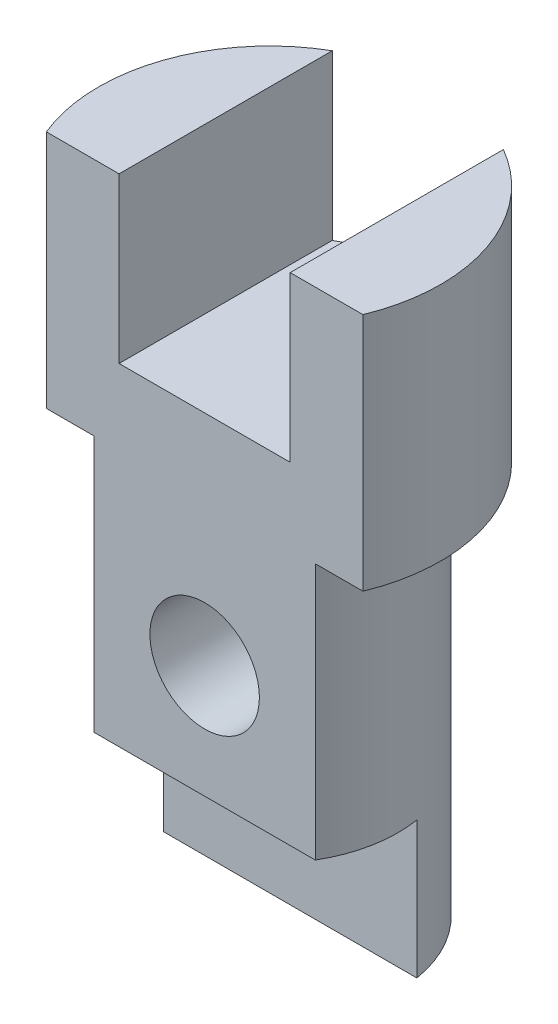
ISO-10303-21;
HEADER;
FILE_DESCRIPTION(('STEP AP214'),'2;1');
FILE_NAME('part.step','',(''),(''),'','','');
FILE_SCHEMA(('AUTOMOTIVE_DESIGN { 1 0 10303 214 1 1 1 1 }'));
ENDSEC;
DATA;
#1=APPLICATION_CONTEXT('core data for automotive mechanical design processes');
#2=APPLICATION_PROTOCOL_DEFINITION('international standard','automotive_design',2000,#1);
#3=PRODUCT_CONTEXT('',#1,'mechanical');
#4=PRODUCT('Part','Part','',(#3));
#5=PRODUCT_RELATED_PRODUCT_CATEGORY('part','',(#4));
#6=PRODUCT_DEFINITION_FORMATION('','',#4);
#7=PRODUCT_DEFINITION_CONTEXT('part definition',#1,'design');
#8=PRODUCT_DEFINITION('design','',#6,#7);
#9=PRODUCT_DEFINITION_SHAPE('','',#8);
#10=(LENGTH_UNIT() NAMED_UNIT(*) SI_UNIT(.MILLI.,.METRE.));
#11=(NAMED_UNIT(*) PLANE_ANGLE_UNIT() SI_UNIT($,.RADIAN.));
#12=(NAMED_UNIT(*) SI_UNIT($,.STERADIAN.) SOLID_ANGLE_UNIT());
#13=UNCERTAINTY_MEASURE_WITH_UNIT(LENGTH_MEASURE(1.E-05),#10,'distance_accuracy_value','');
#14=(GEOMETRIC_REPRESENTATION_CONTEXT(3) GLOBAL_UNCERTAINTY_ASSIGNED_CONTEXT((#13)) GLOBAL_UNIT_ASSIGNED_CONTEXT((#10,
#11,#12)) REPRESENTATION_CONTEXT('',''));
#15=CARTESIAN_POINT('',(0.,0.,0.));
#16=DIRECTION('',(0.,0.,1.));
#17=DIRECTION('',(1.,0.,0.));
#18=AXIS2_PLACEMENT_3D('',#15,#16,#17);
#19=CARTESIAN_POINT('',(0.,0.,0.));
#20=DIRECTION('',(0.,1.,0.));
#21=DIRECTION('',(0.,0.,1.));
#22=AXIS2_PLACEMENT_3D('',#19,#20,#21);
#23=PLANE('',#22);
#24=DIRECTION('',(1.,0.,0.));
#25=VECTOR('',#24,1.);
#26=CARTESIAN_POINT('',(37.5,0.,-6.));
#27=LINE('',#26,#25);
#28=CARTESIAN_POINT('',(-37.0168880377592,0.,-6.));
#29=VERTEX_POINT('',#28);
#30=CARTESIAN_POINT('',(37.0168880377592,0.,-6.));
#31=VERTEX_POINT('',#30);
#32=EDGE_CURVE('E121',#29,#31,#27,.T.);
#33=ORIENTED_EDGE('',*,*,#32,.F.);
#34=CARTESIAN_POINT('',(0.,0.,0.));
#35=DIRECTION('',(0.,1.,0.));
#36=DIRECTION('',(0.,0.,1.));
#37=AXIS2_PLACEMENT_3D('',#34,#35,#36);
#38=CIRCLE('',#37,37.5);
#39=EDGE_CURVE('E147',#31,#29,#38,.T.);
#40=ORIENTED_EDGE('',*,*,#39,.F.);
#41=EDGE_LOOP('',(#33,#40));
#42=FACE_BOUND('',#41,.T.);
#43=ADVANCED_FACE('F39',(#42),#23,.F.);
#44=CARTESIAN_POINT('',(0.,185.,0.));
#45=DIRECTION('',(0.,1.,0.));
#46=DIRECTION('',(0.,0.,1.));
#47=AXIS2_PLACEMENT_3D('',#44,#45,#46);
#48=PLANE('',#47);
#49=DIRECTION('',(0.,0.,1.));
#50=VECTOR('',#49,1.);
#51=CARTESIAN_POINT('',(-25.,185.,0.));
#52=LINE('',#51,#50);
#53=CARTESIAN_POINT('',(-25.,185.,-43.3012701892219));
#54=VERTEX_POINT('',#53);
#55=CARTESIAN_POINT('',(-25.,185.,19.));
#56=VERTEX_POINT('',#55);
#57=EDGE_CURVE('E232',#54,#56,#52,.T.);
#58=ORIENTED_EDGE('',*,*,#57,.F.);
#59=CARTESIAN_POINT('',(0.,185.,0.));
#60=DIRECTION('',(0.,1.,0.));
#61=DIRECTION('',(0.,0.,1.));
#62=AXIS2_PLACEMENT_3D('',#59,#60,#61);
#63=CIRCLE('',#62,50.);
#64=CARTESIAN_POINT('',(-46.2493243193887,185.,19.));
#65=VERTEX_POINT('',#64);
#66=EDGE_CURVE('E151',#54,#65,#63,.T.);
#67=ORIENTED_EDGE('',*,*,#66,.T.);
#68=DIRECTION('',(-1.,0.,0.));
#69=VECTOR('',#68,1.);
#70=CARTESIAN_POINT('',(-81.0320637853745,185.,19.));
#71=LINE('',#70,#69);
#72=EDGE_CURVE('E233',#56,#65,#71,.T.);
#73=ORIENTED_EDGE('',*,*,#72,.F.);
#74=EDGE_LOOP('',(#58,#67,#73));
#75=FACE_BOUND('',#74,.T.);
#76=ADVANCED_FACE('F212',(#75),#48,.T.);
#77=CARTESIAN_POINT('',(0.,115.,0.));
#78=DIRECTION('',(0.,-1.,0.));
#79=DIRECTION('',(0.,0.,-1.));
#80=AXIS2_PLACEMENT_3D('',#77,#78,#79);
#81=CYLINDRICAL_SURFACE('',#80,37.5);
#82=CARTESIAN_POINT('',(0.,89.,-37.5));
#83=CARTESIAN_POINT('',(-0.427809393682003,88.9999969337727,-37.4999975035644));
#84=CARTESIAN_POINT('',(-0.855750855539132,88.9828188276958,-37.4926593971666));
#85=CARTESIAN_POINT('',(-1.70857507942548,88.914269325757,-37.4634893346266));
#86=CARTESIAN_POINT('',(-2.13345581185364,88.8628770348971,-37.4416485215349));
#87=CARTESIAN_POINT('',(-2.97778901536988,88.7262853017906,-37.3839832974588));
#88=CARTESIAN_POINT('',(-3.39722694710041,88.6410092551301,-37.34812720373));
#89=CARTESIAN_POINT('',(-4.22661151459995,88.4375538890515,-37.2633805353818));
#90=CARTESIAN_POINT('',(-4.63655954884625,88.3193794515662,-37.2144918947634));
#91=CARTESIAN_POINT('',(-5.44290236192158,88.0517326400861,-37.1051182322791));
#92=CARTESIAN_POINT('',(-5.83933899573433,87.9023695776649,-37.0446737727429));
#93=CARTESIAN_POINT('',(-6.61771136093352,87.5734153383078,-36.9135705034294));
#94=CARTESIAN_POINT('',(-6.99964659822588,87.3938231325302,-36.8429113460088));
#95=CARTESIAN_POINT('',(-7.7466320543134,87.0059526755,-36.6931156475076));
#96=CARTESIAN_POINT('',(-8.11169147337454,86.7976903068474,-36.613983805453));
#97=CARTESIAN_POINT('',(-8.82337085945239,86.3538043817041,-36.4490277929199));
#98=CARTESIAN_POINT('',(-9.169983537672,86.118170125188,-36.3632010096378));
#99=CARTESIAN_POINT('',(-9.85888463641798,85.6092970979915,-36.1826634377169));
#100=CARTESIAN_POINT('',(-10.2001873828561,85.3348044878858,-36.0877243404792));
#101=CARTESIAN_POINT('',(-10.8587331604742,84.759216877408,-35.8950643354141));
#102=CARTESIAN_POINT('',(-11.1759752405497,84.4581208264345,-35.7973433178287));
#103=CARTESIAN_POINT('',(-11.7848536083808,83.8308975149232,-35.6015385965724));
#104=CARTESIAN_POINT('',(-12.076478449265,83.5047591851922,-35.5034547509695));
#105=CARTESIAN_POINT('',(-12.6323855446282,82.8292527194642,-35.3094822036691));
#106=CARTESIAN_POINT('',(-12.8966632894491,82.4798807676934,-35.2135938660444));
#107=CARTESIAN_POINT('',(-13.4093313695708,81.7408538808232,-35.0216881686697));
#108=CARTESIAN_POINT('',(-13.6561612812667,81.3500472180105,-34.9259278535894));
#109=CARTESIAN_POINT('',(-14.1157132010055,80.5472163133579,-34.7427378989749));
#110=CARTESIAN_POINT('',(-14.3284493772869,80.135200979684,-34.6553048050814));
#111=CARTESIAN_POINT('',(-14.7180272152402,79.292464401259,-34.4916560664736));
#112=CARTESIAN_POINT('',(-14.8948757978245,78.8617467827256,-34.4154382596753));
#113=CARTESIAN_POINT('',(-15.2109072610476,77.9845349036357,-34.2769326880475));
#114=CARTESIAN_POINT('',(-15.3500931001669,77.5380418853839,-34.2146438291393));
#115=CARTESIAN_POINT('',(-15.583229123873,76.6552552785971,-34.1090681440208));
#116=CARTESIAN_POINT('',(-15.6790858493266,76.2195599781898,-34.0649899067631));
#117=CARTESIAN_POINT('',(-15.8342012258165,75.3403624782776,-33.9931671189487));
#118=CARTESIAN_POINT('',(-15.8934610559315,74.8968605307608,-33.9654220421717));
#119=CARTESIAN_POINT('',(-15.9746077788103,74.0059292984363,-33.9273330111729));
#120=CARTESIAN_POINT('',(-15.9965136206885,73.5585021206987,-33.9169802341395));
#121=CARTESIAN_POINT('',(-16.0027173935054,72.6633413005434,-33.9140540684818));
#122=CARTESIAN_POINT('',(-15.9870174519166,72.2156076768949,-33.9214796740808));
#123=CARTESIAN_POINT('',(-15.9210280578624,71.3599452448458,-33.9524965762651));
#124=CARTESIAN_POINT('',(-15.8736526387158,70.9517380290888,-33.9747253938742));
#125=CARTESIAN_POINT('',(-15.7478680268672,70.1411823100594,-34.0332111341828));
#126=CARTESIAN_POINT('',(-15.669460778965,69.7388334412758,-34.069467177777));
#127=CARTESIAN_POINT('',(-15.4823987795988,68.9425843153849,-34.1548807197037));
#128=CARTESIAN_POINT('',(-15.3737395493358,68.5486853185868,-34.2040401283146));
#129=CARTESIAN_POINT('',(-15.1271899097,67.7717846237921,-34.3137918728461));
#130=CARTESIAN_POINT('',(-14.9892983090504,67.3887833706218,-34.374384674689));
#131=CARTESIAN_POINT('',(-14.6821692429184,66.627724243206,-34.5067014461306));
#132=CARTESIAN_POINT('',(-14.512321668075,66.249949621204,-34.5786366978514));
#133=CARTESIAN_POINT('',(-14.1445693088001,65.5098748330488,-34.7306887897201));
#134=CARTESIAN_POINT('',(-13.9466543267551,65.1475803537632,-34.8108086005576));
#135=CARTESIAN_POINT('',(-13.524114495367,64.4403247060522,-34.9771334834255));
#136=CARTESIAN_POINT('',(-13.2994858973421,64.095365980012,-35.0633394088198));
#137=CARTESIAN_POINT('',(-12.8248659101135,63.4244218284922,-35.2397063477261));
#138=CARTESIAN_POINT('',(-12.5748730280777,63.098437521544,-35.3298675938536));
#139=CARTESIAN_POINT('',(-12.0274299761411,62.4387174261641,-35.5201662538126));
#140=CARTESIAN_POINT('',(-11.7277353559451,62.1068904346455,-35.6204753739352));
#141=CARTESIAN_POINT('',(-11.1016838291021,61.4695144099323,-35.8205325955656));
#142=CARTESIAN_POINT('',(-10.7753372170155,61.1639553232707,-35.9202808979301));
#143=CARTESIAN_POINT('',(-10.0974354730267,60.5805842542415,-36.1167051602068));
#144=CARTESIAN_POINT('',(-9.74586326733624,60.3027913754749,-36.2133789740625));
#145=CARTESIAN_POINT('',(-9.01979362267786,59.7771368359943,-36.4010143754922));
#146=CARTESIAN_POINT('',(-8.6453055801583,59.5292630295123,-36.491978273783));
#147=CARTESIAN_POINT('',(-7.86555010793,59.0592106448004,-36.6680637184142));
#148=CARTESIAN_POINT('',(-7.45974033607836,58.837851697203,-36.7529762543261));
#149=CARTESIAN_POINT('',(-6.62871898536882,58.4303660060558,-36.911908962084));
#150=CARTESIAN_POINT('',(-6.20350687047728,58.2442402366346,-36.9859288327565));
#151=CARTESIAN_POINT('',(-5.33688233404436,57.9091616813675,-37.1208820355782));
#152=CARTESIAN_POINT('',(-4.89547760518775,57.7601914996338,-37.1818214899819));
#153=CARTESIAN_POINT('',(-3.99968683731538,57.5009723228447,-37.2888173521372));
#154=CARTESIAN_POINT('',(-3.54530184217216,57.390720223509,-37.3348749530401));
#155=CARTESIAN_POINT('',(-2.65748170218216,57.216184728596,-37.4081941892286));
#156=CARTESIAN_POINT('',(-2.22463085297216,57.14935761735,-37.4364916993181));
#157=CARTESIAN_POINT('',(-1.35419517840626,57.0513970419247,-37.4780730010183));
#158=CARTESIAN_POINT('',(-0.91661056061352,57.0202620190944,-37.4913574482396));
#159=CARTESIAN_POINT('',(-0.04028330680914,56.9940481472324,-37.5025379975856));
#160=CARTESIAN_POINT('',(0.398458994381225,56.9989598177055,-37.5004381458729));
#161=CARTESIAN_POINT('',(1.2737113954877,57.0447599515185,-37.4809185115529));
#162=CARTESIAN_POINT('',(1.71022154930049,57.0856475420309,-37.4634991006201));
#163=CARTESIAN_POINT('',(2.55471094701983,57.1998308833883,-37.4151418322218));
#164=CARTESIAN_POINT('',(2.96298182927553,57.2713059550548,-37.384964446303));
#165=CARTESIAN_POINT('',(3.77166123185948,57.445398457049,-37.3120541209709));
#166=CARTESIAN_POINT('',(4.17207009640244,57.5480145207109,-37.269321732554));
#167=CARTESIAN_POINT('',(4.96249456006103,57.7834392380212,-37.1723314503654));
#168=CARTESIAN_POINT('',(5.35250940760191,57.9162500684229,-37.1180727256739));
#169=CARTESIAN_POINT('',(6.11979465498141,58.2109154578127,-36.9993087681283));
#170=CARTESIAN_POINT('',(6.49706457891802,58.3727710999279,-36.9348031531618));
#171=CARTESIAN_POINT('',(7.24829617701868,58.7297338401958,-36.7948733377872));
#172=CARTESIAN_POINT('',(7.62178813175905,58.9257201820117,-36.7191714619241));
#173=CARTESIAN_POINT('',(8.35095237425475,59.3457464862725,-36.5602360188176));
#174=CARTESIAN_POINT('',(8.70662442784002,59.5697868172376,-36.4770023526398));
#175=CARTESIAN_POINT('',(9.39841022225309,60.0444647504674,-36.304916558195));
#176=CARTESIAN_POINT('',(9.73452015637029,60.2951075028408,-36.2160633433592));
#177=CARTESIAN_POINT('',(10.385586745045,60.8215386575064,-36.0347587855853));
#178=CARTESIAN_POINT('',(10.7005357597546,61.097336057704,-35.9423061619573));
#179=CARTESIAN_POINT('',(11.3303189450724,61.6939928645989,-35.7489903948236));
#180=CARTESIAN_POINT('',(11.6433902375021,62.016679170336,-35.6480145195704));
#181=CARTESIAN_POINT('',(12.2414455857693,62.6874381830647,-35.4470951413787));
#182=CARTESIAN_POINT('',(12.5264277832641,63.0355125670557,-35.3471517071362));
#183=CARTESIAN_POINT('',(13.0666729837597,63.7552918963511,-35.151026944253));
#184=CARTESIAN_POINT('',(13.3219218098313,64.1270079845399,-35.0548474246493));
#185=CARTESIAN_POINT('',(13.8006940386979,64.8917167520828,-34.8691377988472));
#186=CARTESIAN_POINT('',(14.0242300711083,65.2847008748185,-34.7796050523828));
#187=CARTESIAN_POINT('',(14.4415967613811,66.0969282957346,-34.6084106237447));
#188=CARTESIAN_POINT('',(14.6348336798453,66.516512580058,-34.5269156995271));
#189=CARTESIAN_POINT('',(14.9849410341844,67.3727919036068,-34.3764147417215));
#190=CARTESIAN_POINT('',(15.1418107321938,67.8094872897945,-34.3074089615356));
#191=CARTESIAN_POINT('',(15.4173719831434,68.6964960728152,-34.1844617365845));
#192=CARTESIAN_POINT('',(15.5360915309231,69.1467992174891,-34.1305092494583));
#193=CARTESIAN_POINT('',(15.734038406606,70.0576894917864,-34.0397113290951));
#194=CARTESIAN_POINT('',(15.8132697085932,70.5182755816613,-34.0028641744086));
#195=CARTESIAN_POINT('',(15.9264720262152,71.4086194867555,-33.9499784995101));
#196=CARTESIAN_POINT('',(15.9635541216353,71.8378993122814,-33.9325123290704));
#197=CARTESIAN_POINT('',(16.0029528915556,72.6983966947344,-33.9139498439307));
#198=CARTESIAN_POINT('',(16.0052714976181,73.1296141426697,-33.9128526197236));
#199=CARTESIAN_POINT('',(15.9751190490791,73.9904842818431,-33.9270664580879));
#200=CARTESIAN_POINT('',(15.9426533590806,74.4201372041172,-33.942374990484));
#201=CARTESIAN_POINT('',(15.8433360253702,75.2745723719849,-33.9888466891501));
#202=CARTESIAN_POINT('',(15.7764847420453,75.6993546685787,-34.0200096892533));
#203=CARTESIAN_POINT('',(15.6134704900085,76.5192618091907,-34.0951188626737));
#204=CARTESIAN_POINT('',(15.5189867571157,76.914790333569,-34.1383274181644));
#205=CARTESIAN_POINT('',(15.3006886114517,77.6961103264234,-34.2367236617532));
#206=CARTESIAN_POINT('',(15.1768754958735,78.0819022247005,-34.2919108200474));
#207=CARTESIAN_POINT('',(14.9009884727942,78.8415633009056,-34.412689457159));
#208=CARTESIAN_POINT('',(14.7489134720403,79.2154320169543,-34.4782813384473));
#209=CARTESIAN_POINT('',(14.417620020346,79.9494198270715,-34.6181246754593));
#210=CARTESIAN_POINT('',(14.2383909727505,80.3095334843389,-34.6923795092199));
#211=CARTESIAN_POINT('',(13.8422252702114,81.0358110743364,-34.8524200945647));
#212=CARTESIAN_POINT('',(13.6236478498285,81.4009859459006,-34.9386340916045));
#213=CARTESIAN_POINT('',(13.1587855814607,82.1119024367045,-35.1163533076447));
#214=CARTESIAN_POINT('',(12.9124989826985,82.4576428259234,-35.2078588608093));
#215=CARTESIAN_POINT('',(12.3936247754086,83.1280688116129,-35.3938415460716));
#216=CARTESIAN_POINT('',(12.121031059703,83.4527494896935,-35.488319364731));
#217=CARTESIAN_POINT('',(11.5510166119207,84.079416194255,-35.6779237497861));
#218=CARTESIAN_POINT('',(11.2535918258171,84.3813984995483,-35.7730504197788));
#219=CARTESIAN_POINT('',(10.6112596351865,84.9837328822771,-35.9690495146573));
#220=CARTESIAN_POINT('',(10.2644579402489,85.2821121065444,-36.0697897827599));
#221=CARTESIAN_POINT('',(9.54588373802441,85.8485536748473,-36.2665797876147));
#222=CARTESIAN_POINT('',(9.17412023035542,86.1166268527289,-36.3626311935263));
#223=CARTESIAN_POINT('',(8.40738713930146,86.6208112949388,-36.5475230969029));
#224=CARTESIAN_POINT('',(8.01240062603558,86.8568988164076,-36.6363582183671));
#225=CARTESIAN_POINT('',(7.20194480075225,87.2948985194517,-36.8042551589905));
#226=CARTESIAN_POINT('',(6.78647713500349,87.4968134420449,-36.8833177618758));
#227=CARTESIAN_POINT('',(5.94415050303366,87.8618508257115,-37.028326527136));
#228=CARTESIAN_POINT('',(5.51755352946125,88.0255065008251,-37.0944505827829));
#229=CARTESIAN_POINT('',(4.65011384184106,88.3161898957054,-37.2131435123895));
#230=CARTESIAN_POINT('',(4.20926880923362,88.4432116203852,-37.2657101675538));
#231=CARTESIAN_POINT('',(3.31808205333362,88.6588621114293,-37.3555936964116));
#232=CARTESIAN_POINT('',(2.86777016742616,88.7475967217689,-37.392952595242));
#233=CARTESIAN_POINT('',(1.96037804406841,88.8860718156305,-37.4514792964717));
#234=CARTESIAN_POINT('',(1.5033029222712,88.9358403760741,-37.4726587566703));
#235=CARTESIAN_POINT('',(0.871003065462385,88.9772263955303,-37.490288098953));
#236=CARTESIAN_POINT('',(0.696940070310892,88.9857638625143,-37.4939277987901));
#237=CARTESIAN_POINT('',(0.348592025723106,88.997151305371,-37.4987842646913));
#238=CARTESIAN_POINT('',(0.174306975045384,89.0000012493059,-37.5000010171496));
#239=CARTESIAN_POINT('',(0.,89.,-37.5));
#240=B_SPLINE_CURVE_WITH_KNOTS('',3,(#82,#83,#84,#85,#86,#87,#88,#89,#90,#91,#92,#93,#94,#95,
#96,#97,#98,#99,#100,#101,#102,#103,#104,#105,#106,#107,#108,#109,#110,#111,#112,#113,#114,#115,
#116,#117,#118,#119,#120,#121,#122,#123,#124,#125,#126,#127,#128,#129,#130,#131,#132,#133,#134,
#135,#136,#137,#138,#139,#140,#141,#142,#143,#144,#145,#146,#147,#148,#149,#150,#151,#152,#153,
#154,#155,#156,#157,#158,#159,#160,#161,#162,#163,#164,#165,#166,#167,#168,#169,#170,#171,#172,
#173,#174,#175,#176,#177,#178,#179,#180,#181,#182,#183,#184,#185,#186,#187,#188,#189,#190,#191,
#192,#193,#194,#195,#196,#197,#198,#199,#200,#201,#202,#203,#204,#205,#206,#207,#208,#209,#210,
#211,#212,#213,#214,#215,#216,#217,#218,#219,#220,#221,#222,#223,#224,#225,#226,#227,#228,#229,
#230,#231,#232,#233,#234,#235,#236,#237,#238,#239),.UNSPECIFIED.,.T.,.F.,(4,2,2,2,2,2,2,2,2,2,2,
2,2,2,2,2,2,2,2,2,2,2,2,2,2,2,2,2,2,2,2,2,2,2,2,2,2,2,2,2,2,2,2,2,2,2,2,2,2,2,2,2,2,2,2,2,2,2,2,
2,2,2,2,2,2,2,2,2,2,2,2,2,2,2,2,2,2,2,4),(0.,1.28325171569401,2.5672878478366,3.85424359915117,
5.14100847531405,6.42333693288952,7.70570904304405,8.98737358656298,10.2695408461598,
11.6125499995995,12.9556122137859,14.2992715444657,15.6431520986358,17.0575222767648,
18.4713031563329,19.8848111290123,21.298208035687,22.6412631947273,23.9842750809623,
25.3266054746391,26.6688599304373,27.9020565219821,29.1351758399293,30.368477818073,
31.6018300653789,32.8616951963608,34.1220192472005,35.3825203665857,36.6430957167075,
38.0162765461014,39.3889294587302,40.7625203703679,42.1355517783422,43.5437108336608,
44.9519088161442,46.3594462510495,47.7668708087497,49.0818510908885,50.3967739464758,
51.7113509819072,53.0258961246865,54.2711929351168,55.5164351018624,56.761767067108,
58.0071454824069,59.291345014575,60.5755614178931,61.860026894765,63.1449536449793,
64.5257787241736,65.9066950959613,67.2882672194213,68.6692875780881,70.0746757107,
71.4800923551578,72.8844753277411,74.2887169351374,75.5807339494225,76.8726791751577,
78.16442517951,79.4561576456631,80.6816380034519,81.9070641702749,83.1325377500555,
84.358490799062,85.6598115276682,86.9612145251726,88.2629203725296,89.5648391591323,
90.9685326853537,92.371722819916,93.7759488974648,95.1800622872131,96.5632529524803,
97.9466698463939,99.3262374191492,100.704810029641,101.227656119627,101.75050514559),.UNSPECIFIED.);
#241=CARTESIAN_POINT('',(0.,89.,-37.5));
#242=VERTEX_POINT('',#241);
#243=EDGE_CURVE('E187',#242,#242,#240,.T.);
#244=ORIENTED_EDGE('',*,*,#243,.T.);
#245=EDGE_LOOP('',(#244));
#246=FACE_BOUND('',#245,.T.);
#247=CARTESIAN_POINT('',(0.,40.,0.));
#248=DIRECTION('',(0.,1.,0.));
#249=DIRECTION('',(-1.,0.,0.));
#250=AXIS2_PLACEMENT_3D('',#247,#248,#249);
#251=CIRCLE('',#250,37.5);
#252=CARTESIAN_POINT('',(-37.0168880377592,40.,-6.));
#253=VERTEX_POINT('',#252);
#254=CARTESIAN_POINT('',(-32.3303263206544,40.,19.));
#255=VERTEX_POINT('',#254);
#256=EDGE_CURVE('E120',#253,#255,#251,.T.);
#257=ORIENTED_EDGE('',*,*,#256,.T.);
#258=DIRECTION('',(0.,-1.,0.));
#259=VECTOR('',#258,1.);
#260=CARTESIAN_POINT('',(-32.3303263206544,115.,19.));
#261=LINE('',#260,#259);
#262=CARTESIAN_POINT('',(-32.3303263206544,115.,19.));
#263=VERTEX_POINT('',#262);
#264=EDGE_CURVE('E116',#255,#263,#261,.F.);
#265=ORIENTED_EDGE('',*,*,#264,.T.);
#266=CARTESIAN_POINT('',(0.,115.,0.));
#267=DIRECTION('',(0.,1.,0.));
#268=DIRECTION('',(0.,0.,1.));
#269=AXIS2_PLACEMENT_3D('',#266,#267,#268);
#270=CIRCLE('',#269,37.5);
#271=CARTESIAN_POINT('',(32.3303263206544,115.,19.));
#272=VERTEX_POINT('',#271);
#273=EDGE_CURVE('E152',#272,#263,#270,.T.);
#274=ORIENTED_EDGE('',*,*,#273,.F.);
#275=DIRECTION('',(0.,-1.,0.));
#276=VECTOR('',#275,1.);
#277=CARTESIAN_POINT('',(32.3303263206544,115.,19.));
#278=LINE('',#277,#276);
#279=CARTESIAN_POINT('',(32.3303263206544,40.,19.));
#280=VERTEX_POINT('',#279);
#281=EDGE_CURVE('E134',#272,#280,#278,.T.);
#282=ORIENTED_EDGE('',*,*,#281,.T.);
#283=CARTESIAN_POINT('',(37.0168880377592,40.,-6.));
#284=VERTEX_POINT('',#283);
#285=EDGE_CURVE('E54',#280,#284,#251,.T.);
#286=ORIENTED_EDGE('',*,*,#285,.T.);
#287=DIRECTION('',(0.,-1.,0.));
#288=VECTOR('',#287,1.);
#289=CARTESIAN_POINT('',(37.0168880377592,115.,-6.));
#290=LINE('',#289,#288);
#291=EDGE_CURVE('E169',#31,#284,#290,.F.);
#292=ORIENTED_EDGE('',*,*,#291,.F.);
#293=ORIENTED_EDGE('',*,*,#39,.T.);
#294=DIRECTION('',(0.,-1.,0.));
#295=VECTOR('',#294,1.);
#296=CARTESIAN_POINT('',(-37.0168880377592,115.,-6.));
#297=LINE('',#296,#295);
#298=EDGE_CURVE('E123',#253,#29,#297,.T.);
#299=ORIENTED_EDGE('',*,*,#298,.F.);
#300=EDGE_LOOP('',(#257,#265,#274,#282,#286,#292,#293,#299));
#301=FACE_BOUND('',#300,.T.);
#302=ADVANCED_FACE('F41',(#246,#301),#81,.T.);
#303=CARTESIAN_POINT('',(0.,185.,0.));
#304=DIRECTION('',(0.,-1.,0.));
#305=DIRECTION('',(0.,0.,-1.));
#306=AXIS2_PLACEMENT_3D('',#303,#304,#305);
#307=CYLINDRICAL_SURFACE('',#306,50.);
#308=ORIENTED_EDGE('',*,*,#66,.F.);
#309=DIRECTION('',(0.,-1.,0.));
#310=VECTOR('',#309,1.);
#311=CARTESIAN_POINT('',(-25.,185.,-43.3012701892219));
#312=LINE('',#311,#310);
#313=CARTESIAN_POINT('',(-25.,137.,-43.3012701892219));
#314=VERTEX_POINT('',#313);
#315=EDGE_CURVE('E231',#54,#314,#312,.T.);
#316=ORIENTED_EDGE('',*,*,#315,.T.);
#317=CARTESIAN_POINT('',(0.,137.,0.));
#318=DIRECTION('',(0.,-1.,0.));
#319=DIRECTION('',(0.,0.,-1.));
#320=AXIS2_PLACEMENT_3D('',#317,#318,#319);
#321=CIRCLE('',#320,50.);
#322=CARTESIAN_POINT('',(25.,137.,-43.3012701892219));
#323=VERTEX_POINT('',#322);
#324=EDGE_CURVE('E198',#314,#323,#321,.T.);
#325=ORIENTED_EDGE('',*,*,#324,.T.);
#326=DIRECTION('',(0.,-1.,0.));
#327=VECTOR('',#326,1.);
#328=CARTESIAN_POINT('',(25.,185.,-43.301270189222));
#329=LINE('',#328,#327);
#330=CARTESIAN_POINT('',(25.,185.,-43.301270189222));
#331=VERTEX_POINT('',#330);
#332=EDGE_CURVE('E237',#323,#331,#329,.F.);
#333=ORIENTED_EDGE('',*,*,#332,.T.);
#334=CARTESIAN_POINT('',(46.2493243193887,185.,19.));
#335=VERTEX_POINT('',#334);
#336=EDGE_CURVE('E150',#335,#331,#63,.T.);
#337=ORIENTED_EDGE('',*,*,#336,.F.);
#338=DIRECTION('',(0.,-1.,0.));
#339=VECTOR('',#338,1.);
#340=CARTESIAN_POINT('',(46.2493243193887,185.,19.));
#341=LINE('',#340,#339);
#342=CARTESIAN_POINT('',(46.2493243193887,115.,19.));
#343=VERTEX_POINT('',#342);
#344=EDGE_CURVE('E140',#335,#343,#341,.T.);
#345=ORIENTED_EDGE('',*,*,#344,.T.);
#346=CARTESIAN_POINT('',(0.,115.,0.));
#347=DIRECTION('',(0.,1.,0.));
#348=DIRECTION('',(0.,0.,1.));
#349=AXIS2_PLACEMENT_3D('',#346,#347,#348);
#350=CIRCLE('',#349,50.);
#351=CARTESIAN_POINT('',(-46.2493243193887,115.,19.));
#352=VERTEX_POINT('',#351);
#353=EDGE_CURVE('E148',#343,#352,#350,.T.);
#354=ORIENTED_EDGE('',*,*,#353,.T.);
#355=DIRECTION('',(0.,-1.,0.));
#356=VECTOR('',#355,1.);
#357=CARTESIAN_POINT('',(-46.2493243193887,185.,19.));
#358=LINE('',#357,#356);
#359=EDGE_CURVE('E131',#352,#65,#358,.F.);
#360=ORIENTED_EDGE('',*,*,#359,.T.);
#361=EDGE_LOOP('',(#308,#316,#325,#333,#337,#345,#354,#360));
#362=FACE_BOUND('',#361,.T.);
#363=ADVANCED_FACE('F215',(#362),#307,.T.);
#364=DIRECTION('',(0.,0.,-1.));
#365=VECTOR('',#364,1.);
#366=CARTESIAN_POINT('',(25.,185.,0.));
#367=LINE('',#366,#365);
#368=CARTESIAN_POINT('',(25.,185.,19.));
#369=VERTEX_POINT('',#368);
#370=EDGE_CURVE('E244',#369,#331,#367,.T.);
#371=ORIENTED_EDGE('',*,*,#370,.F.);
#372=EDGE_CURVE('E136',#335,#369,#71,.T.);
#373=ORIENTED_EDGE('',*,*,#372,.F.);
#374=ORIENTED_EDGE('',*,*,#336,.T.);
#375=EDGE_LOOP('',(#371,#373,#374));
#376=FACE_BOUND('',#375,.T.);
#377=ADVANCED_FACE('F207',(#376),#48,.T.);
#378=CARTESIAN_POINT('',(0.,115.,0.));
#379=DIRECTION('',(0.,1.,0.));
#380=DIRECTION('',(0.,0.,1.));
#381=AXIS2_PLACEMENT_3D('',#378,#379,#380);
#382=PLANE('',#381);
#383=ORIENTED_EDGE('',*,*,#353,.F.);
#384=DIRECTION('',(-1.,0.,0.));
#385=VECTOR('',#384,1.);
#386=CARTESIAN_POINT('',(0.,115.,19.));
#387=LINE('',#386,#385);
#388=EDGE_CURVE('E160',#343,#272,#387,.T.);
#389=ORIENTED_EDGE('',*,*,#388,.T.);
#390=ORIENTED_EDGE('',*,*,#273,.T.);
#391=EDGE_CURVE('E135',#263,#352,#387,.T.);
#392=ORIENTED_EDGE('',*,*,#391,.T.);
#393=EDGE_LOOP('',(#383,#389,#390,#392));
#394=FACE_BOUND('',#393,.T.);
#395=ADVANCED_FACE('F164',(#394),#382,.F.);
#396=CARTESIAN_POINT('',(-81.0320637853745,-45.0000000000001,19.));
#397=DIRECTION('',(0.,0.,-1.));
#398=DIRECTION('',(-1.,0.,0.));
#399=AXIS2_PLACEMENT_3D('',#396,#397,#398);
#400=PLANE('',#399);
#401=CARTESIAN_POINT('',(0.,73.,19.));
#402=DIRECTION('',(0.,0.,1.));
#403=DIRECTION('',(1.,0.,0.));
#404=AXIS2_PLACEMENT_3D('',#401,#402,#403);
#405=CIRCLE('',#404,16.);
#406=CARTESIAN_POINT('',(16.,73.,19.));
#407=VERTEX_POINT('',#406);
#408=EDGE_CURVE('E179',#407,#407,#405,.T.);
#409=ORIENTED_EDGE('',*,*,#408,.F.);
#410=EDGE_LOOP('',(#409));
#411=FACE_BOUND('',#410,.T.);
#412=ORIENTED_EDGE('',*,*,#264,.F.);
#413=DIRECTION('',(1.,0.,0.));
#414=VECTOR('',#413,1.);
#415=CARTESIAN_POINT('',(-81.0320637853745,40.,19.));
#416=LINE('',#415,#414);
#417=EDGE_CURVE('E11',#255,#280,#416,.T.);
#418=ORIENTED_EDGE('',*,*,#417,.T.);
#419=ORIENTED_EDGE('',*,*,#281,.F.);
#420=ORIENTED_EDGE('',*,*,#388,.F.);
#421=ORIENTED_EDGE('',*,*,#344,.F.);
#422=ORIENTED_EDGE('',*,*,#372,.T.);
#423=DIRECTION('',(0.,1.,0.));
#424=VECTOR('',#423,1.);
#425=CARTESIAN_POINT('',(25.,199.840020356779,19.));
#426=LINE('',#425,#424);
#427=CARTESIAN_POINT('',(25.,137.,19.));
#428=VERTEX_POINT('',#427);
#429=EDGE_CURVE('E185',#428,#369,#426,.T.);
#430=ORIENTED_EDGE('',*,*,#429,.F.);
#431=DIRECTION('',(1.,0.,0.));
#432=VECTOR('',#431,1.);
#433=CARTESIAN_POINT('',(-25.,137.,19.));
#434=LINE('',#433,#432);
#435=CARTESIAN_POINT('',(-25.,137.,19.));
#436=VERTEX_POINT('',#435);
#437=EDGE_CURVE('E176',#436,#428,#434,.T.);
#438=ORIENTED_EDGE('',*,*,#437,.F.);
#439=DIRECTION('',(0.,1.,0.));
#440=VECTOR('',#439,1.);
#441=CARTESIAN_POINT('',(-25.,-45.0000000000001,19.));
#442=LINE('',#441,#440);
#443=EDGE_CURVE('E48',#436,#56,#442,.T.);
#444=ORIENTED_EDGE('',*,*,#443,.T.);
#445=ORIENTED_EDGE('',*,*,#72,.T.);
#446=ORIENTED_EDGE('',*,*,#359,.F.);
#447=ORIENTED_EDGE('',*,*,#391,.F.);
#448=EDGE_LOOP('',(#412,#418,#419,#420,#421,#422,#430,#438,#444,#445,#446,#447));
#449=FACE_BOUND('',#448,.T.);
#450=ADVANCED_FACE('F128',(#411,#449),#400,.F.);
#451=CARTESIAN_POINT('',(0.,73.,-211.));
#452=DIRECTION('',(0.,0.,1.));
#453=DIRECTION('',(1.,0.,0.));
#454=AXIS2_PLACEMENT_3D('',#451,#452,#453);
#455=CYLINDRICAL_SURFACE('',#454,16.);
#456=ORIENTED_EDGE('',*,*,#408,.T.);
#457=EDGE_LOOP('',(#456));
#458=FACE_BOUND('',#457,.T.);
#459=ORIENTED_EDGE('',*,*,#243,.F.);
#460=EDGE_LOOP('',(#459));
#461=FACE_BOUND('',#460,.T.);
#462=ADVANCED_FACE('F196',(#458,#461),#455,.F.);
#463=CARTESIAN_POINT('',(-25.,199.840020356779,-211.));
#464=DIRECTION('',(-1.,0.,0.));
#465=DIRECTION('',(0.,-1.,0.));
#466=AXIS2_PLACEMENT_3D('',#463,#464,#465);
#467=PLANE('',#466);
#468=ORIENTED_EDGE('',*,*,#57,.T.);
#469=ORIENTED_EDGE('',*,*,#443,.F.);
#470=DIRECTION('',(0.,0.,1.));
#471=VECTOR('',#470,1.);
#472=CARTESIAN_POINT('',(-25.,137.,-211.));
#473=LINE('',#472,#471);
#474=EDGE_CURVE('E65',#314,#436,#473,.T.);
#475=ORIENTED_EDGE('',*,*,#474,.F.);
#476=ORIENTED_EDGE('',*,*,#315,.F.);
#477=EDGE_LOOP('',(#468,#469,#475,#476));
#478=FACE_BOUND('',#477,.T.);
#479=ADVANCED_FACE('F201',(#478),#467,.F.);
#480=CARTESIAN_POINT('',(25.,199.840020356779,-211.));
#481=DIRECTION('',(1.,0.,0.));
#482=DIRECTION('',(0.,1.,0.));
#483=AXIS2_PLACEMENT_3D('',#480,#481,#482);
#484=PLANE('',#483);
#485=DIRECTION('',(0.,0.,1.));
#486=VECTOR('',#485,1.);
#487=CARTESIAN_POINT('',(25.,137.,-211.));
#488=LINE('',#487,#486);
#489=EDGE_CURVE('E184',#323,#428,#488,.T.);
#490=ORIENTED_EDGE('',*,*,#489,.T.);
#491=ORIENTED_EDGE('',*,*,#429,.T.);
#492=ORIENTED_EDGE('',*,*,#370,.T.);
#493=ORIENTED_EDGE('',*,*,#332,.F.);
#494=EDGE_LOOP('',(#490,#491,#492,#493));
#495=FACE_BOUND('',#494,.T.);
#496=ADVANCED_FACE('F252',(#495),#484,.F.);
#497=CARTESIAN_POINT('',(-25.,137.,-211.));
#498=DIRECTION('',(0.,-1.,0.));
#499=DIRECTION('',(0.,0.,-1.));
#500=AXIS2_PLACEMENT_3D('',#497,#498,#499);
#501=PLANE('',#500);
#502=ORIENTED_EDGE('',*,*,#474,.T.);
#503=ORIENTED_EDGE('',*,*,#437,.T.);
#504=ORIENTED_EDGE('',*,*,#489,.F.);
#505=ORIENTED_EDGE('',*,*,#324,.F.);
#506=EDGE_LOOP('',(#502,#503,#504,#505));
#507=FACE_BOUND('',#506,.T.);
#508=ADVANCED_FACE('F249',(#507),#501,.F.);
#509=CARTESIAN_POINT('',(0.,0.,-6.));
#510=DIRECTION('',(0.,0.,1.));
#511=DIRECTION('',(1.,0.,0.));
#512=AXIS2_PLACEMENT_3D('',#509,#510,#511);
#513=PLANE('',#512);
#514=ORIENTED_EDGE('',*,*,#298,.T.);
#515=ORIENTED_EDGE('',*,*,#32,.T.);
#516=ORIENTED_EDGE('',*,*,#291,.T.);
#517=DIRECTION('',(-1.,0.,0.));
#518=VECTOR('',#517,1.);
#519=CARTESIAN_POINT('',(37.5,40.,-6.));
#520=LINE('',#519,#518);
#521=EDGE_CURVE('E175',#284,#253,#520,.T.);
#522=ORIENTED_EDGE('',*,*,#521,.T.);
#523=EDGE_LOOP('',(#514,#515,#516,#522));
#524=FACE_BOUND('',#523,.T.);
#525=ADVANCED_FACE('F172',(#524),#513,.T.);
#526=CARTESIAN_POINT('',(37.5,40.,-6.));
#527=DIRECTION('',(0.,1.,0.));
#528=DIRECTION('',(-1.,0.,0.));
#529=AXIS2_PLACEMENT_3D('',#526,#527,#528);
#530=PLANE('',#529);
#531=ORIENTED_EDGE('',*,*,#417,.F.);
#532=ORIENTED_EDGE('',*,*,#256,.F.);
#533=ORIENTED_EDGE('',*,*,#521,.F.);
#534=ORIENTED_EDGE('',*,*,#285,.F.);
#535=EDGE_LOOP('',(#531,#532,#533,#534));
#536=FACE_BOUND('',#535,.T.);
#537=ADVANCED_FACE('F130',(#536),#530,.F.);
#538=CLOSED_SHELL('',(#43,#76,#302,#363,#377,#395,#450,#462,#479,#496,#508,#525,#537));
#539=MANIFOLD_SOLID_BREP('B2',#538);
#540=ADVANCED_BREP_SHAPE_REPRESENTATION('',(#18,#539),#14);
#541=SHAPE_DEFINITION_REPRESENTATION(#9,#540);
ENDSEC;
END-ISO-10303-21;
